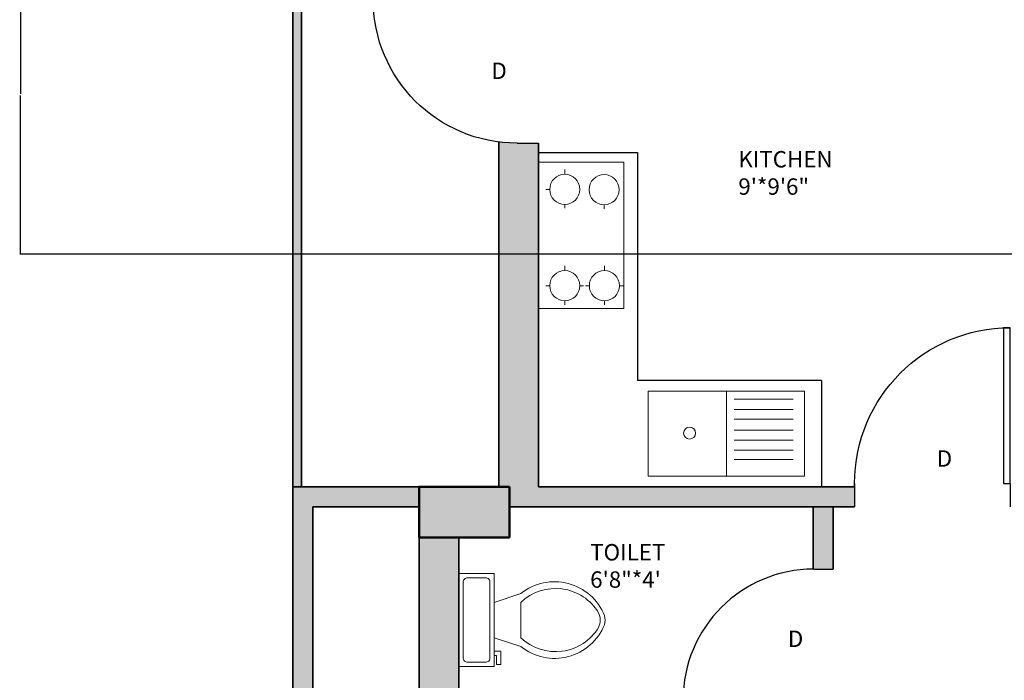
# Model space of a CAD drawing. Units: inches. Extents: x 1998 to 2588, y 1139 to 1977.
# Tile 2 of 134: x 1998 to 2220, y 1427 to 1576. Entities that reach past the tile are written whole.
import ezdxf

# ---------------------------------------------------------------- set-up
doc = ezdxf.new("R2010")
doc.units = ezdxf.units.IN
for name, color, linetype, lineweight in [('A-ANNO-DIMS', 2, 'Continuous', 18), ('A-AREA-IDEN', 7, 'Continuous', 18), ('A-COLS-PATT', 250, 'Continuous', 13), ('A-DOOR-IDEN', 7, 'Continuous', 18), ('A-EQPM', 21, 'Continuous', 18), ('A-FLOR-CASE', 32, 'Continuous', 25), ('A-FLOR-FIXT', 9, 'Continuous', 18), ('A-WALL-PATT', 252, 'Continuous', 13), ('COLUMN', 10, 'Continuous', 50), ('DOOR', 52, 'Continuous', 25), ('WALL', 200, 'Continuous', 35)]:
    doc.layers.add(name, color=color, linetype=linetype, lineweight=lineweight)
doc.styles.get("Standard").update_dxf_attribs({"font": 'arial.ttf'})
doc.dimstyles.get("Standard").update_dxf_attribs({"dimtxt": 0.18, "dimasz": 0.18, "dimexe": 0.18, "dimexo": 0.0625, "dimgap": 0.09, "dimtad": 0, "dimtih": 1, "dimtoh": 1, "dimdec": 4, "dimzin": 0, "dimdsep": 46, "dimtxsty": 'Standard', "dimcen": 0.09, "dimadec": 0, "dimazin": 0, "dimtfac": 1, "dimtdec": 4, "dimtofl": 0, "dimtmove": 0, "dimatfit": 3, "dimfxl": 1, "dimtolj": 1, "dimtzin": 0, "dimarcsym": 0})

# ---------------------------------------------------------------- blocks, each defined once
blk = doc.blocks.new('*U2')
for p, q in [((0, 0), (0, -6)), ((40, 0), (40, -6))]:
    blk.add_line(p, q)
blk.add_lwpolyline([(0, 0), (0, 40), (1.75, 40), (1.75, 0)], close=True)
blk.add_arc((0, 0), 40, 0, 90)
blk = doc.blocks.new('*U4')
for p, q in [((9.5, -6), (9.5, -2)), ((-10, -8.5), (-8, -8.5)), ((-10, -9.5), (-10, -8.5)), ((-8, -8.5), (-8, -8)), ((-7, -8), (-7, -9.5)), ((-4, -8), (-6, -14)), ((4, -8), (6, -14)), ((-7, -9.5), (-10, -9.5)), ((4, -14), (-4, -14))]:
    blk.add_line(p, q)
blk.add_lwpolyline([(10.5, -8), (10.5, 0), (-10.5, 0), (-10.5, -8)], close=True)
for points in [[(-9.5, -2), (-9.5, -6)], [(8.5, -1), (-8.5, -1)], [(-8.5, -7), (8.5, -7)]]:
    blk.add_lwpolyline(points)
for centre, radius, start, end in [((-8.62, -1.88), 0.884, 81.8699, 188.1301), ((8.62, -1.88), 0.884, 351.8699, 98.1301), ((-8.62, -6.12), 0.884, 171.8699, 278.1301), ((8.62, -6.12), 0.884, 261.8699, 8.1301), ((3.52, -21.58), 12.17, 141.4691, 247.9714), ((4.2, -21.82), 11.33, 136.3677, 238.9468), ((-3.52, -21.58), 12.17, 292.0284, 38.5307), ((-4.2, -21.82), 11.33, 301.053, 43.6321), ((0, -27.88), 4, 245.7318, 294.2682), ((0, -29), 4, 254.8605, 285.1395)]:
    blk.add_arc(centre, radius, start, end)
blk = doc.blocks.new('SINK-WITH-DRAINBOARD')
for p, q in [((17.65, 0), (17.65, 19.17)), ((15.93, 17.39), (2.57, 17.39)), ((15.93, 15.02), (2.57, 15.02)), ((15.93, 12.85), (2.57, 12.85)), ((15.93, 10.38), (2.57, 10.38)), ((15.93, 8.14), (2.57, 8.14)), ((15.93, 5.9), (2.57, 5.9)), ((15.93, 3.75), (2.57, 3.75))]:
    blk.add_line(p, q)
blk.add_lwpolyline([(35.31, 19.17), (0, 19.17), (0, 0), (35.31, 0)], close=True)
blk.add_circle((25.96, 9.71), 1.35)
blk = doc.blocks.new('COOKTOP-FOUR-BURNER')
for p, q in [((13.35, 30.32), (13.35, 31.43)), ((16.75, 26.92), (17.59, 26.92)), ((4.47, 23.44), (4.47, 22.56)), ((13.35, 23.52), (13.35, 22.64)), ((4.4, 8.58), (4.4, 9.69)), ((13.35, 8.58), (13.35, 9.69)), ((1, 5.18), (0.17, 5.18)), ((7.8, 5.18), (8.64, 5.18)), ((9.95, 5.18), (9.12, 5.18)), ((16.75, 5.18), (17.59, 5.18)), ((4.4, 1.78), (4.4, 0.89)), ((13.35, 1.78), (13.35, 0.89))]:
    blk.add_line(p, q)
blk.add_lwpolyline([(19.17, 33.08), (0, 33.08), (0, 0), (19.17, 0)], close=True)
for centre in [(4.47, 26.84), (13.35, 26.92), (4.4, 5.18), (13.35, 5.18)]:
    blk.add_circle(centre, 3.4)
blk = doc.blocks.new('*D23')
at = {"layer": 'A-ANNO-DIMS', "color": 0, "lineweight": -2, "transparency": 16777216}
for p, q in [((2549.18, 1476.17), (2549.18, 1138.6)), ((2059.47, 1413.17), (2059.47, 1138.6)), ((2059.65, 1138.78), (2303.93, 1138.78)), ((2549, 1138.78), (2304.72, 1138.78))]:
    blk.add_line(p, q, dxfattribs=at)
at = {"layer": 'A-ANNO-DIMS', "color": 0, "transparency": 16777216}
for points in [[(2059.65, 1138.81), (2059.65, 1138.75), (2059.47, 1138.78)], [(2549, 1138.81), (2549, 1138.75), (2549.18, 1138.78)]]:
    blk.add_solid(points, dxfattribs=at)
at = {"layer": 'Defpoints', "color": 0, "transparency": 16777216}
for p in [(2549.18, 1476.23), (2059.47, 1413.23), (2549.18, 1138.78)]:
    blk.add_point(p, dxfattribs=at)
at = {"layer": 'A-ANNO-DIMS', "color": 0, "transparency": 16777216, "insert": (2304.33, 1138.78), "char_height": 0.18, "attachment_point": 5}
blk.add_mtext('\\A1;489.7', dxfattribs=at)
blk = doc.blocks.new('*D34')
at = {"layer": 'A-ANNO-DIMS', "color": 0, "lineweight": -2, "transparency": 16777216}
for p, q in [((2407.91, 1594.73), (1997.84, 1594.73)), ((1998.02, 1594.55), (1998.02, 1558.91)), ((1998.02, 1522.91), (1998.02, 1558.55)), ((2407.91, 1522.73), (1997.84, 1522.73))]:
    blk.add_line(p, q, dxfattribs=at)
at = {"layer": 'A-ANNO-DIMS', "color": 0, "transparency": 16777216}
for points in [[(1997.99, 1594.55), (1998.05, 1594.55), (1998.02, 1594.73)], [(1997.99, 1522.91), (1998.05, 1522.91), (1998.02, 1522.73)]]:
    blk.add_solid(points, dxfattribs=at)
at = {"layer": 'Defpoints', "color": 0, "transparency": 16777216}
for p in [(1998.02, 1594.73), (2407.97, 1594.73), (2407.97, 1522.73)]:
    blk.add_point(p, dxfattribs=at)
at = {"layer": 'A-ANNO-DIMS', "color": 0, "transparency": 16777216, "insert": (1998.02, 1558.73), "char_height": 0.18, "attachment_point": 5}
blk.add_mtext('\\A1;72', dxfattribs=at)

msp = doc.modelspace()

# ---------------------------------------------------------------- hatches: boundary and pattern name
at = {"layer": 'A-COLS-PATT'}
h = msp.add_hatch(color=256, dxfattribs=at)
h.dxf.hatch_style = 1
h.paths.add_polyline_path([(2099.4125, 1888.7324), (2087.9729, 1888.7324), (2087.9729, 1868.3278), (2099.4125, 1868.3278)])
h.paths.add_polyline_path([(2234.4125, 1888.7324), (2222.9729, 1888.7324), (2222.9729, 1868.3278), (2234.4125, 1868.3278)])
h.paths.add_polyline_path([(2341.4729, 1886.637), (2330.0332, 1886.637), (2330.0332, 1866.2324), (2341.4729, 1866.2324)])
h.paths.add_polyline_path([(2507.8006, 1882.7324), (2487.396, 1882.7324), (2487.396, 1871.2927), (2507.8006, 1871.2927)])
h.paths.add_polyline_path([(2510.9729, 1766.672), (2490.5682, 1766.672), (2490.5682, 1755.2324), (2510.9729, 1755.2324)])
h.paths.add_polyline_path([(2345.9729, 1759.7324), (2334.5332, 1759.7324), (2334.5332, 1739.3278), (2345.9729, 1739.3278)])
h.paths.add_polyline_path([(2234.4125, 1774.3318), (2222.9729, 1774.3318), (2222.9729, 1753.9272), (2234.4125, 1753.9272)])
h.paths.add_polyline_path([(2099.4125, 1775.637), (2087.9729, 1775.637), (2087.9729, 1755.2324), (2099.4125, 1755.2324)])
h.paths.add_polyline_path([(2098.0956, 1593.7241), (2077.691, 1593.7241), (2077.691, 1582.2845), (2098.0956, 1582.2845)])
h.paths.add_polyline_path([(2227.4729, 1604.637), (2216.0332, 1604.637), (2216.0332, 1584.2324), (2227.4729, 1584.2324)])
h.paths.add_polyline_path([(2345.9729, 1647.5211), (2334.5332, 1647.5211), (2334.5332, 1627.1165), (2345.9729, 1627.1165)])
h.paths.add_polyline_path([(2522.3775, 1641.2324), (2501.9729, 1641.2324), (2501.9729, 1629.7927), (2522.3775, 1629.7927)])
h.paths.add_polyline_path([(2522.3775, 1480.7324), (2501.9729, 1480.7324), (2501.9729, 1469.2927), (2522.3775, 1469.2927)])
h.paths.add_polyline_path([(2345.9729, 1488.5616), (2334.5332, 1488.5616), (2334.5332, 1468.1569), (2345.9729, 1468.1569)])
h.paths.add_polyline_path([(2234.4125, 1486.137), (2227.4729, 1486.137), (2227.4729, 1465.7324), (2234.4125, 1465.7324)])
h.paths.add_polyline_path([(2227.4729, 1486.137), (2222.9729, 1486.137), (2222.9729, 1465.7324), (2227.4729, 1465.7324)])
h.paths.add_polyline_path([(2108.3775, 1470.2324), (2087.9729, 1470.2324), (2087.9729, 1458.7927), (2108.3775, 1458.7927)])
h.paths.add_polyline_path([(2096.9729, 1365.5012), (2087.9729, 1365.5012), (2087.9729, 1345.0966), (2096.9729, 1345.0966)])
h.paths.add_polyline_path([(2087.9729, 1365.5012), (2085.5332, 1365.5012), (2085.5332, 1345.0966), (2087.9729, 1345.0966)])
h.paths.add_polyline_path([(2234.4125, 1285.137), (2222.9729, 1285.137), (2222.9729, 1264.7324), (2234.4125, 1264.7324)])
h.paths.add_polyline_path([(2345.9729, 1285.137), (2334.5332, 1285.137), (2334.5332, 1264.7324), (2345.9729, 1264.7324)])
h.paths.add_polyline_path([(2503.1458, 1240.172), (2482.7412, 1240.172), (2482.7412, 1228.7324), (2503.1458, 1228.7324)])
h.paths.add_polyline_path([(2510.9729, 1369.172), (2490.5682, 1369.172), (2490.5682, 1357.7324), (2510.9729, 1357.7324)])
at = {"layer": 'A-WALL-PATT'}
h = msp.add_hatch(color=256, dxfattribs=at)
h.dxf.hatch_style = 1
h.paths.add_polyline_path([(2227.4729, 1911.2324), (2222.9729, 1911.2324), (2222.9729, 1888.7324), (2227.4729, 1888.7324)])
h.paths.add_polyline_path([(2236.4493, 1870.3636), (2236.4493, 1875.2324), (2234.4125, 1875.2324), (2234.4125, 1868.3278), (2227.4729, 1868.3278), (2227.4729, 1866.2324), (2236.4493, 1866.2324)])
h.paths.add_polyline_path([(2330.0332, 1875.2324), (2263.9907, 1875.2324), (2263.9907, 1866.2324), (2330.0332, 1866.2324)])
h.paths.add_polyline_path([(2345.9729, 1906.7324), (2393.9729, 1906.7324), (2393.9729, 1882.7324), (2345.9729, 1882.7324), (2345.9729, 1878.2324), (2393.9729, 1878.2324), (2398.4729, 1878.2324), (2398.4729, 1882.7324), (2398.4729, 1911.2324), (2345.9729, 1911.2324), (2341.4729, 1911.2324), (2341.4729, 1866.2324), (2341.4729, 1790.0412), (2345.9729, 1790.0412), (2345.9729, 1875.2324)])
h.paths.add_polyline_path([(2398.4729, 1878.2324), (2393.9729, 1878.2324), (2393.9729, 1798.2324), (2393.9729, 1793.7324), (2398.4729, 1793.7324)], flags=17)
h.paths.add_polyline_path([(2393.9729, 1798.2324), (2375.7311, 1798.2324, -0.00596797), (2375.7384, 1797.6146), (2375.7384, 1793.7324), (2393.9729, 1793.7324)], flags=17)
h.paths.add_polyline_path([(2349.8569, 1797.6146), (2349.8569, 1798.2324), (2345.9729, 1798.2324), (2345.9729, 1793.7324), (2349.8569, 1793.7324)], flags=17)
h.paths.add_polyline_path([(2398.4729, 1793.7324), (2393.9729, 1793.7324), (2393.9729, 1790.0412), (2398.4729, 1790.0412)], flags=17)
h.paths.add_polyline_path([(2527.4729, 1882.7324), (2507.8006, 1882.7324), (2507.8006, 1878.2324), (2518.4729, 1878.2324), (2518.4729, 1759.7324), (2510.9729, 1759.7324), (2510.9729, 1755.2324), (2527.4729, 1755.2324)])
h.paths.add_polyline_path([(2487.396, 1882.7324), (2398.4729, 1882.7324), (2398.4729, 1878.2324), (2487.396, 1878.2324)])
h.paths.add_polyline_path([(2490.5682, 1759.7324), (2345.9729, 1759.7324), (2345.9729, 1755.2324), (2490.5682, 1755.2324)])
h.paths.add_polyline_path([(2398.4729, 1760.5844), (2398.3914, 1760.5844), (2393.9729, 1760.5844), (2393.9729, 1759.7324), (2398.4729, 1759.7324)])
h.paths.add_polyline_path([(2334.5332, 1759.7324), (2234.4125, 1759.7324), (2234.4125, 1755.2324), (2334.5332, 1755.2324)])
h.paths.add_polyline_path([(2345.9729, 1760.5844), (2341.5543, 1760.5844), (2341.4729, 1760.5844), (2341.4729, 1759.7324), (2345.9729, 1759.7324)])
h.paths.add_polyline_path([(2222.9729, 1759.7324), (2221.7204, 1759.7324), (2221.7204, 1755.2324), (2222.9729, 1755.2324)])
h.paths.add_polyline_path([(2061.4729, 1702.7324), (2059.4729, 1702.7324), (2059.4729, 1584.2324), (2061.4729, 1584.2324)])
h.paths.add_polyline_path([(2061.4729, 1584.2324), (2059.4729, 1584.2324), (2059.4729, 1470.2324), (2061.4729, 1470.2324)])
h.paths.add_polyline_path([(2510.9729, 1469.2927), (2501.9729, 1469.2927), (2501.9729, 1369.172), (2510.9729, 1369.172)])
h.paths.add_polyline_path([(2227.4729, 1369.7324), (2227.4729, 1417.7324), (2221.4126, 1417.7324), (2221.4126, 1413.2324), (2222.9729, 1413.2324), (2222.9729, 1293.2324), (2222.9729, 1285.137), (2227.4729, 1285.137)])
h = msp.add_hatch(color=256, dxfattribs=at)
h.dxf.hatch_style = 1
h.paths.add_polyline_path([(2222.9729, 1888.7324), (2099.4125, 1888.7324), (2099.4125, 1879.7324), (2222.9729, 1879.7324)])
h.paths.add_polyline_path([(2096.9729, 1868.3278), (2087.9729, 1868.3278), (2087.9729, 1775.637), (2096.9729, 1775.637)])
h.paths.add_polyline_path([(2227.4729, 1868.3278), (2222.9729, 1868.3278), (2222.9729, 1774.3318), (2227.4729, 1774.3318)])
h.paths.add_polyline_path([(2188.3019, 1759.7324), (2138.6074, 1759.7324), (2099.4125, 1759.7324), (2099.4125, 1755.2324), (2176.9729, 1755.2324), (2188.3019, 1755.2324)])
h.paths.add_polyline_path([(2087.9729, 1759.7324), (2059.4729, 1759.7324), (2059.4729, 1702.7324), (2087.9729, 1702.7324), (2087.9729, 1707.2324), (2063.9729, 1707.2324), (2063.9729, 1755.2324), (2087.9729, 1755.2324)])
h.paths.add_polyline_path([(2096.9729, 1755.2324), (2087.9729, 1755.2324), (2087.9729, 1707.2324), (2096.9729, 1707.2324)])
h.paths.add_polyline_path([(2187.0461, 1707.2324), (2105.9729, 1707.2324), (2096.9729, 1707.2324), (2087.9729, 1707.2324), (2087.9729, 1702.7324), (2105.9729, 1702.7324), (2114.9729, 1702.7324), (2187.0461, 1702.7324)])
h.paths.add_polyline_path([(2181.4729, 1719.2028), (2176.9729, 1719.2028), (2176.9729, 1707.2324), (2181.4729, 1707.2324)])
h.paths.add_polyline_path([(2216.0332, 1588.7324), (2114.9729, 1588.7324), (2105.9729, 1588.7324), (2105.9729, 1584.2324), (2216.0332, 1584.2324)])
h.paths.add_polyline_path([(2077.691, 1588.7324), (2061.4729, 1588.7324), (2061.4729, 1584.2324), (2077.691, 1584.2324)])
h.paths.add_polyline_path([(2105.9729, 1588.7324), (2098.0956, 1588.7324), (2098.0956, 1584.2324), (2105.9729, 1584.2324)])
h.paths.add_polyline_path([(2114.9729, 1596.2642), (2110.1012, 1596.2642), (2105.9729, 1596.2642), (2105.9729, 1588.7324), (2114.9729, 1588.7324)])
h.paths.add_polyline_path([(2114.9729, 1584.2324), (2105.9729, 1584.2324), (2105.9729, 1580.249), (2110.1012, 1580.249), (2114.9729, 1580.249)])
h.paths.add_polyline_path([(2114.9729, 1547.7716), (2110.1012, 1547.7716, -0.0318759), (2105.9729, 1548.035), (2105.9729, 1470.2324), (2108.3775, 1470.2324), (2108.3775, 1465.7324), (2186.2943, 1465.7324), (2186.2943, 1470.2324), (2114.9729, 1470.2324)])
h.paths.add_polyline_path([(2227.4729, 1584.2324), (2222.9729, 1584.2324), (2222.9729, 1486.137), (2227.4729, 1486.137)])
h.paths.add_polyline_path([(2295.4138, 1593.2324), (2227.4729, 1593.2324), (2227.4729, 1588.7324), (2295.4138, 1588.7324), (2295.4138, 1591.8729)])
h.paths.add_polyline_path([(2345.9729, 1627.1165), (2341.4729, 1627.1165), (2341.4729, 1593.2324), (2337.2869, 1593.2324), (2337.2869, 1591.8729), (2337.2869, 1588.7324), (2345.9729, 1588.7324)])
h.paths.add_polyline_path([(2291.9729, 1588.7324), (2287.4729, 1588.7324), (2287.4729, 1522.7324), (2291.9729, 1522.7324)])
h.paths.add_polyline_path([(2291.9729, 1522.7324), (2287.4729, 1522.7324), (2227.4729, 1522.7324), (2227.4729, 1518.2324), (2291.9729, 1518.2324)])
h.paths.add_polyline_path([(2295.7347, 1519.5919), (2295.7347, 1522.7324), (2291.9729, 1522.7324), (2291.9729, 1518.2324), (2295.7347, 1518.2324)])
h.paths.add_polyline_path([(2345.9729, 1522.7324), (2337.6078, 1522.7324), (2337.6078, 1519.5919), (2337.6078, 1518.2324), (2341.4729, 1518.2324), (2341.4729, 1488.5616), (2345.9729, 1488.5616)])
h.paths.add_polyline_path([(2345.9729, 1468.1569), (2341.4729, 1468.1569), (2341.4729, 1374.2324), (2227.4729, 1374.2324), (2227.4729, 1369.7324), (2345.9729, 1369.7324)])
h.paths.add_polyline_path([(2345.9729, 1369.7324), (2341.4729, 1369.7324), (2341.4729, 1362.2324), (2345.9729, 1362.2324)])
h.paths.add_polyline_path([(2345.9729, 1317.7324), (2345.9729, 1322.2324), (2341.4729, 1322.2324), (2341.4729, 1285.137), (2345.9729, 1285.137)], flags=17)
h.paths.add_polyline_path([(2356.2096, 1322.2324), (2345.9729, 1322.2324), (2345.9729, 1317.7324), (2356.2096, 1317.7324), (2356.2096, 1319.3088)], flags=17)
h.paths.add_polyline_path([(2393.9729, 1322.2324), (2375.6999, 1322.2324), (2375.6999, 1319.3088, -0.02024576), (2375.636, 1317.7324), (2393.9729, 1317.7324)], flags=17)
h.paths.add_polyline_path([(2398.4729, 1322.2324), (2393.9729, 1322.2324), (2393.9729, 1317.7324), (2393.9729, 1237.7324), (2345.9729, 1237.7324), (2345.9729, 1264.7324), (2341.4729, 1264.7324), (2341.4729, 1228.7324), (2393.9729, 1228.7324), (2482.7412, 1228.7324), (2482.7412, 1237.7324), (2398.4729, 1237.7324), (2398.4729, 1297.1029)])
h.paths.add_polyline_path([(2398.4729, 1362.2324), (2393.9729, 1362.2324), (2393.9729, 1357.7324), (2398.4729, 1357.7324)])
h.paths.add_polyline_path([(2345.9729, 1329.7549), (2341.4729, 1329.7549), (2341.4729, 1322.2324), (2345.9729, 1322.2324)])
h = msp.add_hatch(color=256, dxfattribs=at)
h.dxf.hatch_style = 1
h.paths.add_polyline_path([(2527.4729, 1362.2324), (2510.9729, 1362.2324), (2510.9729, 1357.7324), (2518.4729, 1357.7324), (2518.4729, 1237.7324), (2503.1458, 1237.7324), (2503.1458, 1228.7324), (2527.4729, 1228.7324)])
h.paths.add_polyline_path([(2490.5682, 1362.2324), (2398.4729, 1362.2324), (2398.4729, 1357.7324), (2490.5682, 1357.7324)])
h.paths.add_polyline_path([(2224.9729, 1264.7324), (2222.9729, 1264.7324), (2222.9729, 1232.4125), (2341.4729, 1232.4125), (2341.4729, 1234.4125), (2224.9729, 1234.4125)])
h.paths.add_polyline_path([(2334.5332, 1273.7324), (2264.7638, 1273.7324), (2264.7638, 1269.5611, -0.043659), (2264.3413, 1264.7324), (2334.5332, 1264.7324)])
h.paths.add_polyline_path([(2236.9551, 1273.7324), (2234.4125, 1273.7324), (2234.4125, 1264.7324), (2236.9551, 1264.7324), (2236.9551, 1269.5611)])
h.paths.add_polyline_path([(2222.9729, 1293.2324), (2096.9729, 1293.2324), (2096.9729, 1345.0966), (2087.9729, 1345.0966), (2087.9729, 1284.2324), (2222.9729, 1284.2324), (2222.9729, 1285.137)])
h.paths.add_polyline_path([(2096.9729, 1458.7927), (2087.9729, 1458.7927), (2087.9729, 1417.7324), (2087.9729, 1413.2324), (2096.9729, 1413.2324), (2096.9729, 1417.7324)])
h.paths.add_polyline_path([(2096.9729, 1413.2324), (2087.9729, 1413.2324), (2087.9729, 1365.5012), (2096.9729, 1365.5012), (2096.9729, 1369.3358)])
h.paths.add_polyline_path([(2186.2943, 1417.7324), (2138.6074, 1417.7324), (2096.9729, 1417.7324), (2096.9729, 1413.2324), (2138.6074, 1413.2324), (2186.2943, 1413.2324)])
h.paths.add_polyline_path([(2181.4729, 1465.7324), (2176.9729, 1465.7324), (2176.9729, 1451.6434), (2181.4729, 1451.6434)])
h.paths.add_polyline_path([(2181.4729, 1422.1664), (2176.9729, 1422.1664), (2176.9729, 1417.7324), (2181.4729, 1417.7324)])
h.paths.add_polyline_path([(2063.9729, 1465.7324), (2087.9729, 1465.7324), (2087.9729, 1470.2324), (2059.4729, 1470.2324), (2059.4729, 1413.2324), (2087.9729, 1413.2324), (2087.9729, 1417.7324), (2063.9729, 1417.7324)])
h.paths.add_polyline_path([(2181.4729, 1755.2324), (2176.9729, 1755.2324), (2176.9729, 1748.6798), (2177.0513, 1748.6798), (2181.4729, 1748.6798)])
h.paths.add_polyline_path([(2227.4729, 1707.2324), (2220.4647, 1707.2324), (2220.4647, 1702.7324), (2222.9729, 1702.7324), (2222.9729, 1604.637), (2227.4729, 1604.637)])
h.paths.add_polyline_path([(2114.9729, 1702.7324), (2105.9729, 1702.7324), (2105.9729, 1628.4781, -0.0318759), (2110.1012, 1628.7416), (2114.9729, 1628.7416)])
h.paths.add_polyline_path([(2345.9729, 1739.3278), (2341.4729, 1739.3278), (2341.4729, 1647.5211), (2345.9729, 1647.5211)])
h.paths.add_polyline_path([(2350.6273, 1641.2324), (2345.9729, 1641.2324), (2345.9729, 1636.7324), (2350.6273, 1636.7324), (2350.6273, 1639.8729)])
h.paths.add_polyline_path([(2501.9729, 1641.2324), (2407.9729, 1641.2324), (2392.5005, 1641.2324), (2392.5005, 1639.8729), (2392.5005, 1636.7324), (2501.9729, 1636.7324)])
h.paths.add_polyline_path([(2510.9729, 1755.2324), (2501.9729, 1755.2324), (2501.9729, 1641.2324), (2510.9729, 1641.2324)])
h.paths.add_polyline_path([(2549.1786, 1641.2324), (2522.3775, 1641.2324), (2522.3775, 1636.7324), (2540.1786, 1636.7324), (2540.1786, 1480.7324), (2522.3775, 1480.7324), (2522.3775, 1476.2324), (2549.1786, 1476.2324)])
h.paths.add_polyline_path([(2498.1786, 1594.7324), (2407.9729, 1594.7324), (2407.9729, 1585.7324), (2416.9729, 1585.7324), (2489.1786, 1585.7324), (2489.1786, 1531.7324), (2416.9729, 1531.7324), (2407.9729, 1531.7324), (2407.9729, 1522.7324), (2498.1786, 1522.7324)])
h.paths.add_polyline_path([(2351.6437, 1480.7324), (2345.9729, 1480.7324), (2345.9729, 1476.2324), (2351.6437, 1476.2324), (2351.6437, 1477.5919)])
h.paths.add_polyline_path([(2501.9729, 1480.7324), (2498.1786, 1480.7324), (2407.9729, 1480.7324), (2393.5168, 1480.7324), (2393.5168, 1477.5919), (2393.5168, 1476.2324), (2501.9729, 1476.2324)])

# ---------------------------------------------------------------- linework, layer by layer
at = {"layer": 'A-FLOR-CASE'}
for p, q in [((2114.9729, 1545.666), (2114.9729, 1545.666)), ((2114.9729, 1545.666), (2137.2992, 1545.666)), ((2137.2992, 1545.666), (2137.2992, 1494.2324)), ((2178.8044, 1494.2324), (2137.2992, 1494.2324)), ((2178.8044, 1494.2324), (2178.8044, 1470.2324))]:
    msp.add_line(p, q, dxfattribs=at)
at = {"layer": 'COLUMN'}
msp.add_lwpolyline([(2108.3775, 1470.2324), (2108.3775, 1458.7927), (2087.9729, 1458.7927), (2087.9729, 1470.2324)], close=True, dxfattribs=at)
at = {"layer": 'WALL'}
for p, q in [((2061.4729, 1473.2749), (2061.4729, 1705.7749)), ((2059.4729, 1470.2324), (2059.4729, 1702.7324)), ((2105.9729, 1470.2324), (2105.9729, 1548.035)), ((2114.9729, 1470.2324), (2114.9729, 1547.7716)), ((2061.4729, 1473.2749), (2061.4729, 1470.2324)), ((2059.4729, 1470.2324), (2087.9729, 1470.2324)), ((2059.4729, 1413.2324), (2059.4729, 1470.2324)), ((2087.9729, 1417.7324), (2087.9729, 1470.2324)), ((2105.9729, 1470.2324), (2087.9729, 1470.2324)), ((2186.2943, 1470.2324), (2114.9729, 1470.2324)), ((2186.2943, 1470.2324), (2186.2943, 1471.0001)), ((2063.9729, 1417.7324), (2063.9729, 1465.7324)), ((2063.9729, 1465.7324), (2087.9729, 1465.7324)), ((2186.2943, 1465.7324), (2108.3775, 1465.7324)), ((2176.9729, 1451.6433), (2176.9729, 1465.7324)), ((2181.4729, 1451.6434), (2181.4729, 1465.7324)), ((2096.9729, 1417.7324), (2096.9729, 1458.7927))]:
    msp.add_line(p, q, dxfattribs=at)
msp.add_lwpolyline([(2059.4729, 1470.2324), (2061.4729, 1470.2324), (2061.4729, 1584.2324), (2059.4729, 1584.2324)], close=True, dxfattribs=at)

# ---------------------------------------------------------------- block references
at = {"layer": 'A-EQPM', "extrusion": (0, 0, -1), "zscale": -1}
msp.add_blockref('COOKTOP-FOUR-BURNER', (-2134.2201, 1510.426), dxfattribs=at)
at = {"layer": 'A-FLOR-FIXT', "extrusion": (0, 0, -1), "zscale": -1}
msp.add_blockref('SINK-WITH-DRAINBOARD', (-2175.0121, 1472.619), dxfattribs=at)
at = {"layer": 'A-FLOR-FIXT', "rotation": 90.00000000000003}
msp.add_blockref('*U4', (2096.9729, 1440.1452), dxfattribs=at)
at = {"layer": 'DOOR', "rotation": 90}
for p, xscale, yscale, zscale in [((2110.1012, 1580.249), -0.8119355758402486, 0.8119355758402486, 0.8119355758402486), ((2177.0513, 1422.1664), 0.736924595324625, 0.736924595324625, 0.736924595324625)]:
    msp.add_blockref('*U2', p, dxfattribs=dict(at, xscale=xscale, yscale=yscale, zscale=zscale))
at = {"layer": 'DOOR', "xscale": -0.877957807115804, "yscale": 0.877957807115804, "zscale": 0.877957807115804}
msp.add_blockref('*U2', (2221.4126, 1471.0001), dxfattribs=at)

# ---------------------------------------------------------------- texts
at = {"layer": 'A-AREA-IDEN', "char_height": 3.69875, "attachment_point": 1}
for s, insert in [('KITCHEN\\P9\'*9\'6"', (2160.0515, 1545.9927)), ('TOILET\\P6\'8"*4\'', (2126.6028, 1457.2994))]:
    msp.add_mtext_dynamic_manual_height_columns(s, width=110.572713, gutter_width=18.4938, heights=[0], dxfattribs=dict(at, insert=insert))
at = {"layer": 'A-DOOR-IDEN', "char_height": 3.6988, "attachment_point": 1}
for insert in [(2104.3181, 1565.9515), (2204.8377, 1478.4576), (2171.2322, 1437.7707)]:
    msp.add_mtext_dynamic_manual_height_columns('D', width=110.572713, gutter_width=18.4938, heights=[0], dxfattribs=dict(at, insert=insert))

# ---------------------------------------------------------------- dimensions: what is measured, and where the dimension line sits
at = {"layer": 'A-ANNO-DIMS'}
dim = msp.add_linear_dim(base=(1998.0229, 1594.7324), p1=(2407.9729, 1522.7324), p2=(2407.9729, 1594.7324), angle=90, dimstyle='Standard', override={"dimdec": 0, "dimlfac": 1, "dimrnd": 0, "dimzin": 0, "dimdsep": 46, "dimlunit": 2}, dxfattribs=at)
dim.commit()
dim.dimension.update_dxf_attribs({"geometry": '*D34', "text_midpoint": (1998.0229, 1558.7324)})
dim = msp.add_linear_dim(base=(2549.1786, 1138.7824), p1=(2059.4729, 1413.2324), p2=(2549.1786, 1476.2324), dimstyle='Standard', override={"dimdec": 1, "dimlfac": 1, "dimrnd": 0, "dimzin": 0, "dimdsep": 46, "dimlunit": 2}, dxfattribs=at)
dim.commit()
dim.dimension.update_dxf_attribs({"geometry": '*D23', "text_midpoint": (2304.3257, 1138.7824)})

doc.saveas('drawing.dxf')
